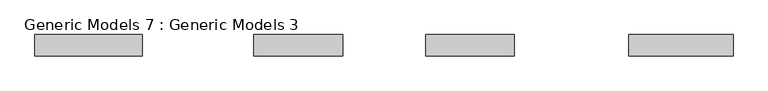
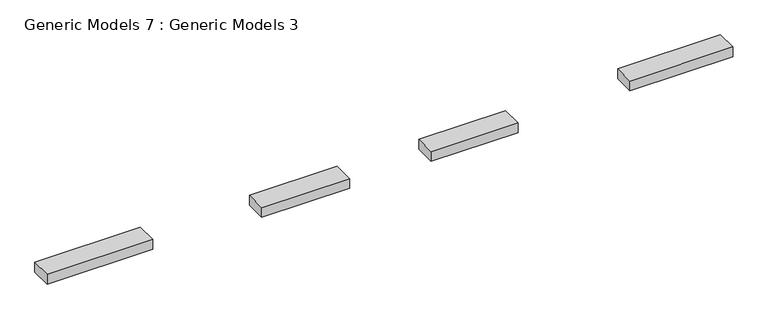
"""IFC4 building model written with IfcOpenShell, lengths in millimetres: proxy geometry, Generic Models 7 : Generic Models 3."""

from ifc_helpers import new_model, si_unit, frame, origin, place, context, project, spatial, polyline, outline, extrude, source, transform, mapped, element, save


def generic_models_7_generic_models_3_e4b45389(model_context):
    return source(origin(), model_context, "Body", "SweptSolid", [
        extrude(outline(polyline([(-6067.1942397, 8885.5272103), (-4578.5596144, 8885.5272103), (-4578.5596144, 8580.7272103), (-6067.1942397, 8580.7272103), (-6067.1942397, 8885.5272103)])), frame((0.0, 0.0, 5613.4), z_axis=(0.0, 0.0, 1.0), x_axis=(1.0, 0.0, 0.0)), (0.0, 0.0, 1.0), 152.4),
        extrude(outline(polyline([(-8952.7187727, 8885.5272103), (-7692.9270478, 8885.5272103), (-7692.9270478, 8580.7272103), (-8952.7187727, 8580.7272103), (-8952.7187727, 8885.5272103)])), frame((0.0, 0.0, 5543.55), z_axis=(0.0, 0.0, 1.0), x_axis=(1.0, 0.0, 0.0)), (0.0, 0.0, 1.0), 152.4),
        extrude(outline(polyline([(-11403.4518443, 8885.5272103), (-10134.7895677, 8885.5272103), (-10134.7895677, 8580.7272103), (-11403.4518443, 8580.7272103), (-11403.4518443, 8885.5272103)])), frame((0.0, 0.0, 5543.55), z_axis=(0.0, 0.0, 1.0), x_axis=(1.0, 0.0, 0.0)), (0.0, 0.0, 1.0), 152.4),
        extrude(outline(polyline([(-14517.0685074, 8885.5272103), (-12988.5597404, 8885.5272103), (-12988.5597404, 8580.7272103), (-14517.0685074, 8580.7272103), (-14517.0685074, 8885.5272103)])), frame((0.0, 0.0, 5613.4), z_axis=(0.0, 0.0, 1.0), x_axis=(1.0, 0.0, 0.0)), (0.0, 0.0, 1.0), 152.4),
    ])


if __name__ == "__main__":
    model = new_model("IFC4")
    model_context = context("Model", 3, world=origin())
    ifc_project = project(units=[si_unit("LENGTHUNIT", "METRE", prefix="MILLI")], contexts=[model_context])
    site = spatial("IfcSite", under=ifc_project)
    building = spatial("IfcBuilding", under=site)
    placement = place(None, origin())
    generic_models_7_generic_models_3_shape = generic_models_7_generic_models_3_e4b45389(model_context)
    element("IfcBuildingElementProxy", 1, Name="Generic Models 7 : Generic Models 3", ObjectType="Generic Models 7 : Generic Models 3", at=placement, inside=building, context=model_context, shape_type="MappedRepresentation", body=[
        mapped(generic_models_7_generic_models_3_shape, transform((0.0, 0.0, 0.0), x_axis=(1.0, 0.0, 0.0), y_axis=(0.0, 1.0, 0.0), z_axis=(0.0, 0.0, 1.0))),
    ])
    save(model, "model.ifc")
